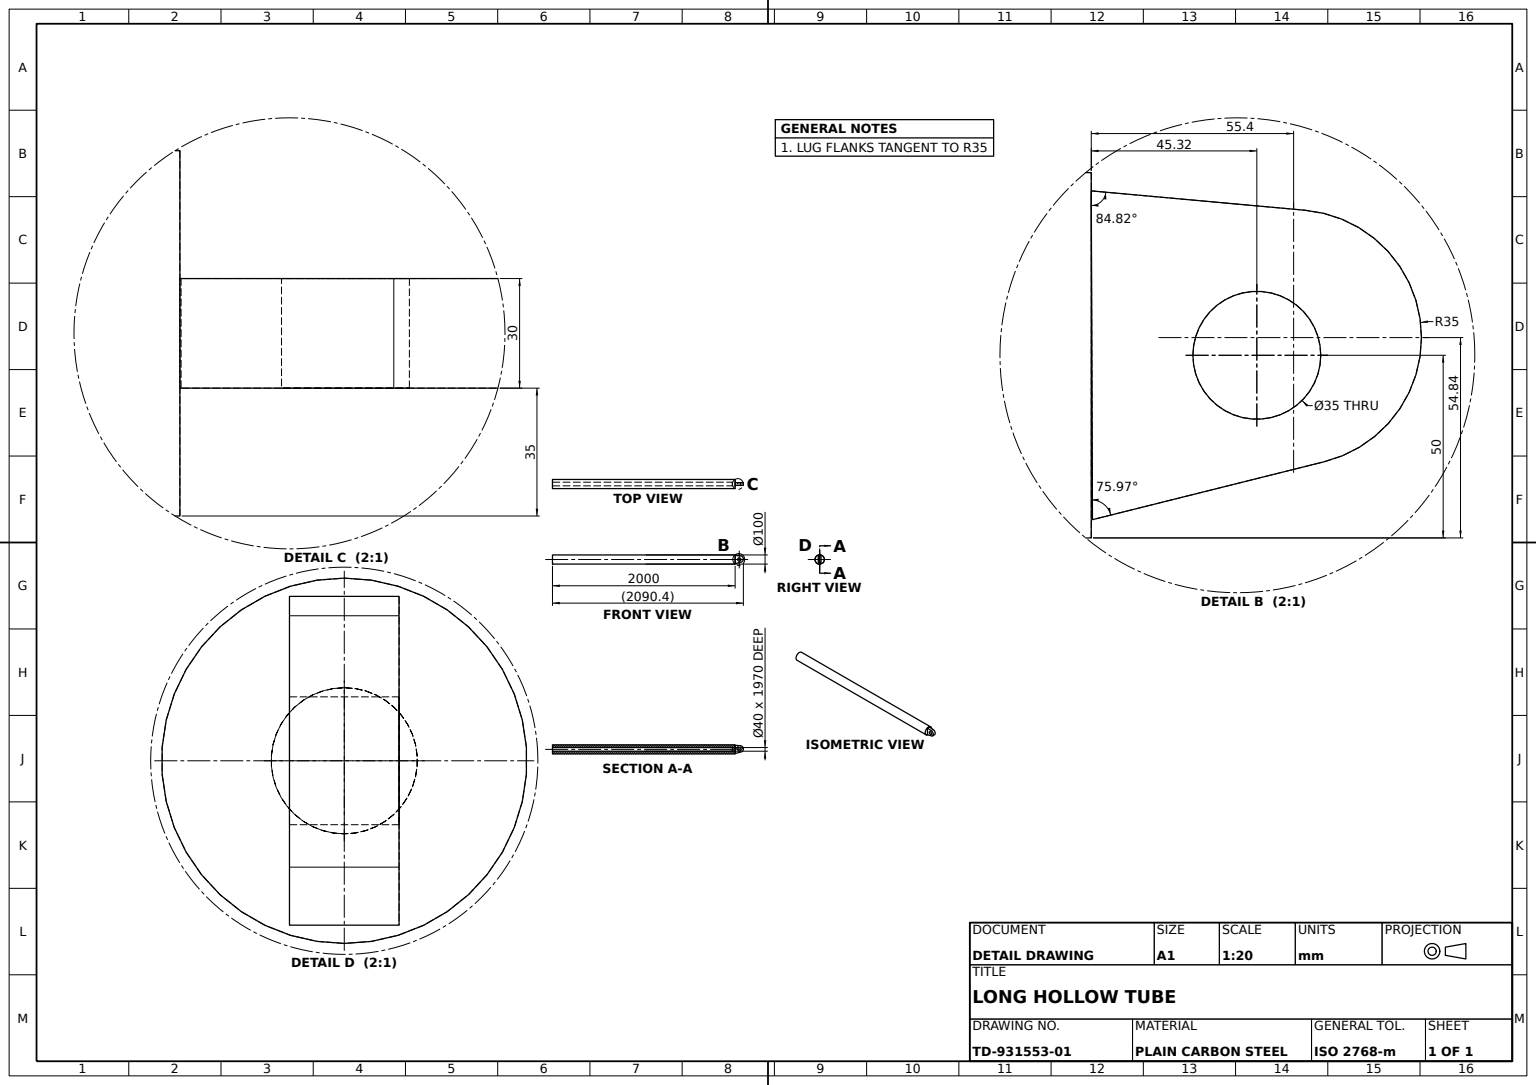
from build123d import *

# Parameters (mm, degrees)
TUBE_PROFILE_100_R     = 50
TUBE_100X2000_DEPTH    = 2000
TUBE_SHELL_30_WALL_T   = -30
EYE_LUG_PROFILE_R      = 17.5
EYE_LUG_30_THICK_DEPTH = 15


with BuildPart() as part:
    # Tube Profile Ø100 → Tube Ø100x2000 (new body)
    with BuildSketch(Plane.XY):
        Circle(TUBE_PROFILE_100_R)
    extrude(amount=TUBE_100X2000_DEPTH)

    # Tube Shell 30 Wall
    tube_shell_30_wall_openings = [part.faces().sort_by_distance(p)[0] for p in [
        (0, 0, 2000),
    ]]
    offset(amount=TUBE_SHELL_30_WALL_T, openings=tube_shell_30_wall_openings, kind=Kind.INTERSECTION)


with BuildPart() as body_2:
    # Eye Lug Profile → Eye Lug 30 Thick (new, symmetric)
    with BuildSketch(Plane(origin=(0, 0, 0), x_dir=(1, 0, 0), z_dir=(0, 1, 0))):
        with BuildLine():
            Line((-45, 0), (-39.695897674, 58.555029213))
            ThreePointArc((-39.695897674, 58.555029213), (-7.540074868, 90.293133194), (29.117384917, 63.882248566))
            Line((29.117384917, 63.882248566), (44.998831412, 0.324301638))
            Line((44.998831412, 0.324301638), (-45, 0))
        make_face()
        with Locations(Location((0, 45.324301638, 0), (0, 0, 270))):
            Circle(EYE_LUG_PROFILE_R, mode=Mode.SUBTRACT)
    extrude(amount=EYE_LUG_30_THICK_DEPTH, both=True)


solid = Compound([part.part, body_2.part])
